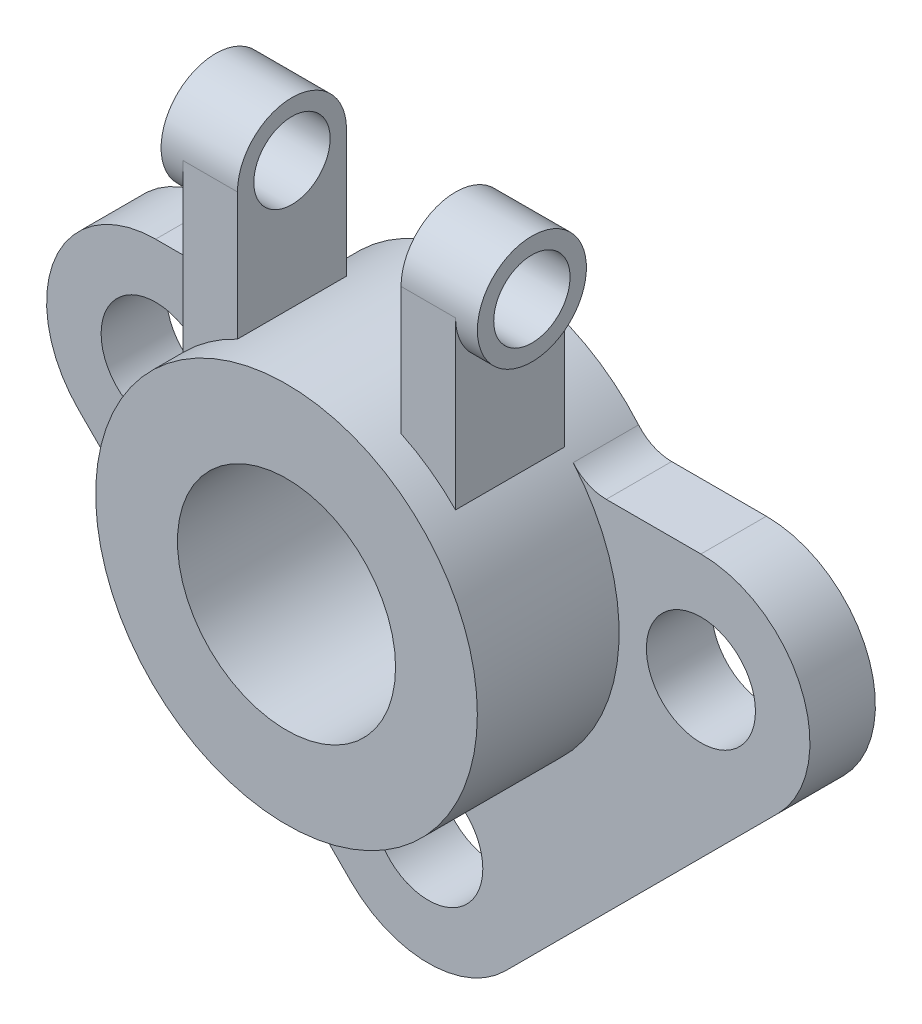
ISO-10303-21;
HEADER;
FILE_DESCRIPTION(('STEP AP214'),'2;1');
FILE_NAME('part.step','',(''),(''),'','','');
FILE_SCHEMA(('AUTOMOTIVE_DESIGN { 1 0 10303 214 1 1 1 1 }'));
ENDSEC;
DATA;
#1=APPLICATION_CONTEXT('core data for automotive mechanical design processes');
#2=APPLICATION_PROTOCOL_DEFINITION('international standard','automotive_design',2000,#1);
#3=PRODUCT_CONTEXT('',#1,'mechanical');
#4=PRODUCT('Part','Part','',(#3));
#5=PRODUCT_RELATED_PRODUCT_CATEGORY('part','',(#4));
#6=PRODUCT_DEFINITION_FORMATION('','',#4);
#7=PRODUCT_DEFINITION_CONTEXT('part definition',#1,'design');
#8=PRODUCT_DEFINITION('design','',#6,#7);
#9=PRODUCT_DEFINITION_SHAPE('','',#8);
#10=(LENGTH_UNIT() NAMED_UNIT(*) SI_UNIT(.MILLI.,.METRE.));
#11=(NAMED_UNIT(*) PLANE_ANGLE_UNIT() SI_UNIT($,.RADIAN.));
#12=(NAMED_UNIT(*) SI_UNIT($,.STERADIAN.) SOLID_ANGLE_UNIT());
#13=UNCERTAINTY_MEASURE_WITH_UNIT(LENGTH_MEASURE(1.E-05),#10,'distance_accuracy_value','');
#14=(GEOMETRIC_REPRESENTATION_CONTEXT(3) GLOBAL_UNCERTAINTY_ASSIGNED_CONTEXT((#13)) GLOBAL_UNIT_ASSIGNED_CONTEXT((#10,
#11,#12)) REPRESENTATION_CONTEXT('',''));
#15=CARTESIAN_POINT('',(0.,0.,0.));
#16=DIRECTION('',(0.,0.,1.));
#17=DIRECTION('',(1.,0.,0.));
#18=AXIS2_PLACEMENT_3D('',#15,#16,#17);
#19=CARTESIAN_POINT('',(0.,0.,38.));
#20=DIRECTION('',(0.,0.,-1.));
#21=DIRECTION('',(-1.,0.,0.));
#22=AXIS2_PLACEMENT_3D('',#19,#20,#21);
#23=CYLINDRICAL_SURFACE('',#22,35.);
#24=CARTESIAN_POINT('',(0.,0.,32.));
#25=DIRECTION('',(0.,0.,1.));
#26=DIRECTION('',(1.,0.,0.));
#27=AXIS2_PLACEMENT_3D('',#24,#25,#26);
#28=CIRCLE('',#27,35.);
#29=CARTESIAN_POINT('',(25.,24.4948974278318,32.));
#30=VERTEX_POINT('',#29);
#31=CARTESIAN_POINT('',(15.,31.6227766016838,32.));
#32=VERTEX_POINT('',#31);
#33=EDGE_CURVE('E309',#30,#32,#28,.T.);
#34=ORIENTED_EDGE('',*,*,#33,.T.);
#35=DIRECTION('',(0.,0.,-1.));
#36=VECTOR('',#35,1.);
#37=CARTESIAN_POINT('',(15.,31.6227766016838,38.));
#38=LINE('',#37,#36);
#39=CARTESIAN_POINT('',(15.,31.6227766016838,12.));
#40=VERTEX_POINT('',#39);
#41=EDGE_CURVE('E11',#32,#40,#38,.T.);
#42=ORIENTED_EDGE('',*,*,#41,.T.);
#43=CARTESIAN_POINT('',(0.,0.,12.));
#44=DIRECTION('',(0.,0.,-1.));
#45=DIRECTION('',(-1.,0.,0.));
#46=AXIS2_PLACEMENT_3D('',#43,#44,#45);
#47=CIRCLE('',#46,35.);
#48=CARTESIAN_POINT('',(25.,24.4948974278318,12.));
#49=VERTEX_POINT('',#48);
#50=EDGE_CURVE('E50',#40,#49,#47,.T.);
#51=ORIENTED_EDGE('',*,*,#50,.T.);
#52=DIRECTION('',(0.,0.,-1.));
#53=VECTOR('',#52,1.);
#54=CARTESIAN_POINT('',(25.,24.4948974278318,38.));
#55=LINE('',#54,#53);
#56=EDGE_CURVE('E311',#49,#30,#55,.F.);
#57=ORIENTED_EDGE('',*,*,#56,.T.);
#58=EDGE_LOOP('',(#34,#42,#51,#57));
#59=FACE_BOUND('',#58,.T.);
#60=CARTESIAN_POINT('',(0.,0.,12.));
#61=DIRECTION('',(0.,0.,-1.));
#62=DIRECTION('',(-1.,0.,0.));
#63=AXIS2_PLACEMENT_3D('',#60,#61,#62);
#64=CIRCLE('',#63,35.);
#65=CARTESIAN_POINT('',(-25.,24.4948974278318,12.));
#66=VERTEX_POINT('',#65);
#67=CARTESIAN_POINT('',(-15.,31.6227766016838,12.));
#68=VERTEX_POINT('',#67);
#69=EDGE_CURVE('E301',#66,#68,#64,.T.);
#70=ORIENTED_EDGE('',*,*,#69,.T.);
#71=DIRECTION('',(0.,0.,-1.));
#72=VECTOR('',#71,1.);
#73=CARTESIAN_POINT('',(-15.,31.6227766016838,38.));
#74=LINE('',#73,#72);
#75=CARTESIAN_POINT('',(-15.,31.6227766016838,32.));
#76=VERTEX_POINT('',#75);
#77=EDGE_CURVE('E177',#68,#76,#74,.F.);
#78=ORIENTED_EDGE('',*,*,#77,.T.);
#79=CARTESIAN_POINT('',(0.,0.,32.));
#80=DIRECTION('',(0.,0.,1.));
#81=DIRECTION('',(1.,0.,0.));
#82=AXIS2_PLACEMENT_3D('',#79,#80,#81);
#83=CIRCLE('',#82,35.);
#84=CARTESIAN_POINT('',(-25.,24.4948974278318,32.));
#85=VERTEX_POINT('',#84);
#86=EDGE_CURVE('E308',#76,#85,#83,.T.);
#87=ORIENTED_EDGE('',*,*,#86,.T.);
#88=DIRECTION('',(0.,0.,-1.));
#89=VECTOR('',#88,1.);
#90=CARTESIAN_POINT('',(-25.,24.4948974278318,38.));
#91=LINE('',#90,#89);
#92=EDGE_CURVE('E302',#85,#66,#91,.T.);
#93=ORIENTED_EDGE('',*,*,#92,.T.);
#94=EDGE_LOOP('',(#70,#78,#87,#93));
#95=FACE_BOUND('',#94,.T.);
#96=CARTESIAN_POINT('',(0.,0.,38.));
#97=DIRECTION('',(0.,0.,1.));
#98=DIRECTION('',(1.,0.,0.));
#99=AXIS2_PLACEMENT_3D('',#96,#97,#98);
#100=CIRCLE('',#99,35.);
#101=CARTESIAN_POINT('',(35.,0.,38.));
#102=VERTEX_POINT('',#101);
#103=EDGE_CURVE('E277',#102,#102,#100,.T.);
#104=ORIENTED_EDGE('',*,*,#103,.F.);
#105=EDGE_LOOP('',(#104));
#106=FACE_BOUND('',#105,.T.);
#107=CARTESIAN_POINT('',(0.,0.,0.));
#108=DIRECTION('',(0.,0.,1.));
#109=DIRECTION('',(1.,0.,0.));
#110=AXIS2_PLACEMENT_3D('',#107,#108,#109);
#111=CIRCLE('',#110,35.);
#112=CARTESIAN_POINT('',(26.5628330475733,22.7906976744186,0.));
#113=VERTEX_POINT('',#112);
#114=CARTESIAN_POINT('',(-26.5628330475733,22.7906976744186,0.));
#115=VERTEX_POINT('',#114);
#116=EDGE_CURVE('E272',#113,#115,#111,.T.);
#117=ORIENTED_EDGE('',*,*,#116,.T.);
#118=DIRECTION('',(0.,0.,-1.));
#119=VECTOR('',#118,1.);
#120=CARTESIAN_POINT('',(-26.5628330475733,22.7906976744186,38.));
#121=LINE('',#120,#119);
#122=CARTESIAN_POINT('',(-26.5628330475733,22.7906976744186,12.));
#123=VERTEX_POINT('',#122);
#124=EDGE_CURVE('E290',#115,#123,#121,.F.);
#125=ORIENTED_EDGE('',*,*,#124,.T.);
#126=CARTESIAN_POINT('',(0.,0.,12.));
#127=DIRECTION('',(0.,0.,-1.));
#128=DIRECTION('',(1.,0.,0.));
#129=AXIS2_PLACEMENT_3D('',#126,#127,#128);
#130=CIRCLE('',#129,35.);
#131=CARTESIAN_POINT('',(26.5628330475733,22.7906976744186,12.));
#132=VERTEX_POINT('',#131);
#133=EDGE_CURVE('E223',#132,#123,#130,.T.);
#134=ORIENTED_EDGE('',*,*,#133,.F.);
#135=DIRECTION('',(0.,0.,-1.));
#136=VECTOR('',#135,1.);
#137=CARTESIAN_POINT('',(26.5628330475733,22.7906976744186,38.));
#138=LINE('',#137,#136);
#139=EDGE_CURVE('E284',#132,#113,#138,.T.);
#140=ORIENTED_EDGE('',*,*,#139,.T.);
#141=EDGE_LOOP('',(#117,#125,#134,#140));
#142=FACE_BOUND('',#141,.T.);
#143=ADVANCED_FACE('F39',(#59,#95,#106,#142),#23,.T.);
#144=CARTESIAN_POINT('',(0.,0.,38.));
#145=DIRECTION('',(0.,0.,1.));
#146=DIRECTION('',(1.,0.,0.));
#147=AXIS2_PLACEMENT_3D('',#144,#145,#146);
#148=PLANE('',#147);
#149=ORIENTED_EDGE('',*,*,#103,.T.);
#150=EDGE_LOOP('',(#149));
#151=FACE_BOUND('',#150,.T.);
#152=CARTESIAN_POINT('',(0.,0.,38.));
#153=DIRECTION('',(0.,0.,1.));
#154=DIRECTION('',(1.,0.,0.));
#155=AXIS2_PLACEMENT_3D('',#152,#153,#154);
#156=CIRCLE('',#155,20.);
#157=CARTESIAN_POINT('',(20.,0.,38.));
#158=VERTEX_POINT('',#157);
#159=EDGE_CURVE('E269',#158,#158,#156,.T.);
#160=ORIENTED_EDGE('',*,*,#159,.F.);
#161=EDGE_LOOP('',(#160));
#162=FACE_BOUND('',#161,.T.);
#163=ADVANCED_FACE('F368',(#151,#162),#148,.T.);
#164=CARTESIAN_POINT('',(0.,0.,0.));
#165=DIRECTION('',(0.,0.,1.));
#166=DIRECTION('',(1.,0.,0.));
#167=AXIS2_PLACEMENT_3D('',#164,#165,#166);
#168=PLANE('',#167);
#169=ORIENTED_EDGE('',*,*,#116,.F.);
#170=CARTESIAN_POINT('',(32.6343377441615,28.,0.));
#171=DIRECTION('',(0.,0.,1.));
#172=DIRECTION('',(1.,0.,0.));
#173=AXIS2_PLACEMENT_3D('',#170,#171,#172);
#174=CIRCLE('',#173,8.);
#175=CARTESIAN_POINT('',(32.6343377441615,20.,0.));
#176=VERTEX_POINT('',#175);
#177=EDGE_CURVE('E297',#113,#176,#174,.T.);
#178=ORIENTED_EDGE('',*,*,#177,.T.);
#179=DIRECTION('',(-1.,0.,0.));
#180=VECTOR('',#179,1.);
#181=CARTESIAN_POINT('',(50.,20.,0.));
#182=LINE('',#181,#180);
#183=CARTESIAN_POINT('',(50.,20.,0.));
#184=VERTEX_POINT('',#183);
#185=EDGE_CURVE('E238',#184,#176,#182,.T.);
#186=ORIENTED_EDGE('',*,*,#185,.F.);
#187=CARTESIAN_POINT('',(50.,0.,0.));
#188=DIRECTION('',(0.,0.,1.));
#189=DIRECTION('',(1.,0.,0.));
#190=AXIS2_PLACEMENT_3D('',#187,#188,#189);
#191=CIRCLE('',#190,20.);
#192=CARTESIAN_POINT('',(64.142135623731,-14.1421356237309,0.));
#193=VERTEX_POINT('',#192);
#194=EDGE_CURVE('E214',#193,#184,#191,.T.);
#195=ORIENTED_EDGE('',*,*,#194,.F.);
#196=DIRECTION('',(0.707106781186547,0.707106781186548,0.));
#197=VECTOR('',#196,1.);
#198=CARTESIAN_POINT('',(14.142135623731,-64.142135623731,0.));
#199=LINE('',#198,#197);
#200=CARTESIAN_POINT('',(14.1421356237309,-64.142135623731,0.));
#201=VERTEX_POINT('',#200);
#202=EDGE_CURVE('E225',#201,#193,#199,.T.);
#203=ORIENTED_EDGE('',*,*,#202,.F.);
#204=CARTESIAN_POINT('',(0.,-50.,0.));
#205=DIRECTION('',(0.,0.,1.));
#206=DIRECTION('',(1.,0.,0.));
#207=AXIS2_PLACEMENT_3D('',#204,#205,#206);
#208=CIRCLE('',#207,20.);
#209=CARTESIAN_POINT('',(-14.142135623731,-64.142135623731,0.));
#210=VERTEX_POINT('',#209);
#211=EDGE_CURVE('E248',#210,#201,#208,.T.);
#212=ORIENTED_EDGE('',*,*,#211,.F.);
#213=DIRECTION('',(0.707106781186547,-0.707106781186547,0.));
#214=VECTOR('',#213,1.);
#215=CARTESIAN_POINT('',(-64.142135623731,-14.142135623731,0.));
#216=LINE('',#215,#214);
#217=CARTESIAN_POINT('',(-64.142135623731,-14.142135623731,0.));
#218=VERTEX_POINT('',#217);
#219=EDGE_CURVE('E250',#218,#210,#216,.T.);
#220=ORIENTED_EDGE('',*,*,#219,.F.);
#221=CARTESIAN_POINT('',(-50.,0.,0.));
#222=DIRECTION('',(0.,0.,1.));
#223=DIRECTION('',(-1.,0.,0.));
#224=AXIS2_PLACEMENT_3D('',#221,#222,#223);
#225=CIRCLE('',#224,20.);
#226=CARTESIAN_POINT('',(-50.,20.,0.));
#227=VERTEX_POINT('',#226);
#228=EDGE_CURVE('E241',#227,#218,#225,.T.);
#229=ORIENTED_EDGE('',*,*,#228,.F.);
#230=DIRECTION('',(-1.,0.,0.));
#231=VECTOR('',#230,1.);
#232=CARTESIAN_POINT('',(-50.,20.,0.));
#233=LINE('',#232,#231);
#234=CARTESIAN_POINT('',(-32.6343377441615,20.,0.));
#235=VERTEX_POINT('',#234);
#236=EDGE_CURVE('E243',#235,#227,#233,.T.);
#237=ORIENTED_EDGE('',*,*,#236,.F.);
#238=CARTESIAN_POINT('',(-32.6343377441615,28.,0.));
#239=DIRECTION('',(0.,0.,1.));
#240=DIRECTION('',(1.,0.,0.));
#241=AXIS2_PLACEMENT_3D('',#238,#239,#240);
#242=CIRCLE('',#241,8.);
#243=EDGE_CURVE('E295',#235,#115,#242,.T.);
#244=ORIENTED_EDGE('',*,*,#243,.T.);
#245=EDGE_LOOP('',(#169,#178,#186,#195,#203,#212,#220,#229,#237,#244));
#246=FACE_BOUND('',#245,.T.);
#247=CARTESIAN_POINT('',(0.,0.,0.));
#248=DIRECTION('',(0.,0.,1.));
#249=DIRECTION('',(1.,0.,0.));
#250=AXIS2_PLACEMENT_3D('',#247,#248,#249);
#251=CIRCLE('',#250,20.);
#252=CARTESIAN_POINT('',(20.,0.,0.));
#253=VERTEX_POINT('',#252);
#254=EDGE_CURVE('E267',#253,#253,#251,.T.);
#255=ORIENTED_EDGE('',*,*,#254,.T.);
#256=EDGE_LOOP('',(#255));
#257=FACE_BOUND('',#256,.T.);
#258=CARTESIAN_POINT('',(50.,0.,0.));
#259=DIRECTION('',(0.,0.,1.));
#260=DIRECTION('',(1.,0.,0.));
#261=AXIS2_PLACEMENT_3D('',#258,#259,#260);
#262=CIRCLE('',#261,10.);
#263=CARTESIAN_POINT('',(60.,0.,0.));
#264=VERTEX_POINT('',#263);
#265=EDGE_CURVE('E207',#264,#264,#262,.T.);
#266=ORIENTED_EDGE('',*,*,#265,.T.);
#267=EDGE_LOOP('',(#266));
#268=FACE_BOUND('',#267,.T.);
#269=CARTESIAN_POINT('',(0.,-50.,0.));
#270=DIRECTION('',(0.,0.,1.));
#271=DIRECTION('',(1.,0.,0.));
#272=AXIS2_PLACEMENT_3D('',#269,#270,#271);
#273=CIRCLE('',#272,10.);
#274=CARTESIAN_POINT('',(10.,-50.,0.));
#275=VERTEX_POINT('',#274);
#276=EDGE_CURVE('E201',#275,#275,#273,.T.);
#277=ORIENTED_EDGE('',*,*,#276,.T.);
#278=EDGE_LOOP('',(#277));
#279=FACE_BOUND('',#278,.T.);
#280=CARTESIAN_POINT('',(-50.,0.,0.));
#281=DIRECTION('',(0.,0.,1.));
#282=DIRECTION('',(-1.,0.,0.));
#283=AXIS2_PLACEMENT_3D('',#280,#281,#282);
#284=CIRCLE('',#283,10.);
#285=CARTESIAN_POINT('',(-60.,0.,0.));
#286=VERTEX_POINT('',#285);
#287=EDGE_CURVE('E194',#286,#286,#284,.T.);
#288=ORIENTED_EDGE('',*,*,#287,.T.);
#289=EDGE_LOOP('',(#288));
#290=FACE_BOUND('',#289,.T.);
#291=ADVANCED_FACE('F375',(#246,#257,#268,#279,#290),#168,.F.);
#292=CARTESIAN_POINT('',(0.,0.,38.));
#293=DIRECTION('',(0.,0.,-1.));
#294=DIRECTION('',(-1.,0.,0.));
#295=AXIS2_PLACEMENT_3D('',#292,#293,#294);
#296=CYLINDRICAL_SURFACE('',#295,20.);
#297=ORIENTED_EDGE('',*,*,#159,.T.);
#298=EDGE_LOOP('',(#297));
#299=FACE_BOUND('',#298,.T.);
#300=ORIENTED_EDGE('',*,*,#254,.F.);
#301=EDGE_LOOP('',(#300));
#302=FACE_BOUND('',#301,.T.);
#303=ADVANCED_FACE('F432',(#299,#302),#296,.F.);
#304=CARTESIAN_POINT('',(50.,0.,12.));
#305=DIRECTION('',(0.,0.,1.));
#306=DIRECTION('',(1.,0.,0.));
#307=AXIS2_PLACEMENT_3D('',#304,#305,#306);
#308=PLANE('',#307);
#309=CARTESIAN_POINT('',(0.,-50.,12.));
#310=DIRECTION('',(0.,0.,1.));
#311=DIRECTION('',(1.,0.,0.));
#312=AXIS2_PLACEMENT_3D('',#309,#310,#311);
#313=CIRCLE('',#312,10.);
#314=CARTESIAN_POINT('',(10.,-50.,12.));
#315=VERTEX_POINT('',#314);
#316=EDGE_CURVE('E206',#315,#315,#313,.T.);
#317=ORIENTED_EDGE('',*,*,#316,.F.);
#318=EDGE_LOOP('',(#317));
#319=FACE_BOUND('',#318,.T.);
#320=CARTESIAN_POINT('',(50.,0.,12.));
#321=DIRECTION('',(0.,0.,1.));
#322=DIRECTION('',(1.,0.,0.));
#323=AXIS2_PLACEMENT_3D('',#320,#321,#322);
#324=CIRCLE('',#323,20.);
#325=CARTESIAN_POINT('',(64.142135623731,-14.1421356237309,12.));
#326=VERTEX_POINT('',#325);
#327=CARTESIAN_POINT('',(50.,20.,12.));
#328=VERTEX_POINT('',#327);
#329=EDGE_CURVE('E217',#326,#328,#324,.T.);
#330=ORIENTED_EDGE('',*,*,#329,.T.);
#331=DIRECTION('',(-1.,0.,0.));
#332=VECTOR('',#331,1.);
#333=CARTESIAN_POINT('',(50.,20.,12.));
#334=LINE('',#333,#332);
#335=CARTESIAN_POINT('',(32.6343377441615,20.,12.));
#336=VERTEX_POINT('',#335);
#337=EDGE_CURVE('E222',#328,#336,#334,.T.);
#338=ORIENTED_EDGE('',*,*,#337,.T.);
#339=CARTESIAN_POINT('',(32.6343377441615,28.,12.));
#340=DIRECTION('',(0.,0.,1.));
#341=DIRECTION('',(1.,0.,0.));
#342=AXIS2_PLACEMENT_3D('',#339,#340,#341);
#343=CIRCLE('',#342,8.);
#344=EDGE_CURVE('E298',#336,#132,#343,.F.);
#345=ORIENTED_EDGE('',*,*,#344,.T.);
#346=ORIENTED_EDGE('',*,*,#133,.T.);
#347=CARTESIAN_POINT('',(-32.6343377441615,28.,12.));
#348=DIRECTION('',(0.,0.,1.));
#349=DIRECTION('',(1.,0.,0.));
#350=AXIS2_PLACEMENT_3D('',#347,#348,#349);
#351=CIRCLE('',#350,8.);
#352=CARTESIAN_POINT('',(-32.6343377441615,20.,12.));
#353=VERTEX_POINT('',#352);
#354=EDGE_CURVE('E294',#123,#353,#351,.F.);
#355=ORIENTED_EDGE('',*,*,#354,.T.);
#356=DIRECTION('',(-1.,0.,0.));
#357=VECTOR('',#356,1.);
#358=CARTESIAN_POINT('',(-50.,20.,12.));
#359=LINE('',#358,#357);
#360=CARTESIAN_POINT('',(-50.,20.,12.));
#361=VERTEX_POINT('',#360);
#362=EDGE_CURVE('E230',#353,#361,#359,.T.);
#363=ORIENTED_EDGE('',*,*,#362,.T.);
#364=CARTESIAN_POINT('',(-50.,0.,12.));
#365=DIRECTION('',(0.,0.,1.));
#366=DIRECTION('',(-1.,0.,0.));
#367=AXIS2_PLACEMENT_3D('',#364,#365,#366);
#368=CIRCLE('',#367,20.);
#369=CARTESIAN_POINT('',(-64.142135623731,-14.142135623731,12.));
#370=VERTEX_POINT('',#369);
#371=EDGE_CURVE('E229',#361,#370,#368,.T.);
#372=ORIENTED_EDGE('',*,*,#371,.T.);
#373=DIRECTION('',(0.707106781186547,-0.707106781186547,0.));
#374=VECTOR('',#373,1.);
#375=CARTESIAN_POINT('',(-64.142135623731,-14.142135623731,12.));
#376=LINE('',#375,#374);
#377=CARTESIAN_POINT('',(-14.142135623731,-64.142135623731,12.));
#378=VERTEX_POINT('',#377);
#379=EDGE_CURVE('E231',#370,#378,#376,.T.);
#380=ORIENTED_EDGE('',*,*,#379,.T.);
#381=CARTESIAN_POINT('',(0.,-50.,12.));
#382=DIRECTION('',(0.,0.,1.));
#383=DIRECTION('',(1.,0.,0.));
#384=AXIS2_PLACEMENT_3D('',#381,#382,#383);
#385=CIRCLE('',#384,20.);
#386=CARTESIAN_POINT('',(14.1421356237309,-64.142135623731,12.));
#387=VERTEX_POINT('',#386);
#388=EDGE_CURVE('E232',#378,#387,#385,.T.);
#389=ORIENTED_EDGE('',*,*,#388,.T.);
#390=DIRECTION('',(0.707106781186547,0.707106781186548,0.));
#391=VECTOR('',#390,1.);
#392=CARTESIAN_POINT('',(14.142135623731,-64.142135623731,12.));
#393=LINE('',#392,#391);
#394=EDGE_CURVE('E234',#387,#326,#393,.T.);
#395=ORIENTED_EDGE('',*,*,#394,.T.);
#396=EDGE_LOOP('',(#330,#338,#345,#346,#355,#363,#372,#380,#389,#395));
#397=FACE_BOUND('',#396,.T.);
#398=CARTESIAN_POINT('',(50.,0.,12.));
#399=DIRECTION('',(0.,0.,1.));
#400=DIRECTION('',(1.,0.,0.));
#401=AXIS2_PLACEMENT_3D('',#398,#399,#400);
#402=CIRCLE('',#401,10.);
#403=CARTESIAN_POINT('',(60.,0.,12.));
#404=VERTEX_POINT('',#403);
#405=EDGE_CURVE('E215',#404,#404,#402,.T.);
#406=ORIENTED_EDGE('',*,*,#405,.F.);
#407=EDGE_LOOP('',(#406));
#408=FACE_BOUND('',#407,.T.);
#409=CARTESIAN_POINT('',(-50.,0.,12.));
#410=DIRECTION('',(0.,0.,1.));
#411=DIRECTION('',(-1.,0.,0.));
#412=AXIS2_PLACEMENT_3D('',#409,#410,#411);
#413=CIRCLE('',#412,10.);
#414=CARTESIAN_POINT('',(-60.,0.,12.));
#415=VERTEX_POINT('',#414);
#416=EDGE_CURVE('E199',#415,#415,#413,.T.);
#417=ORIENTED_EDGE('',*,*,#416,.F.);
#418=EDGE_LOOP('',(#417));
#419=FACE_BOUND('',#418,.T.);
#420=ADVANCED_FACE('F393',(#319,#397,#408,#419),#308,.T.);
#421=CARTESIAN_POINT('',(50.,0.,12.));
#422=DIRECTION('',(0.,0.,-1.));
#423=DIRECTION('',(-1.,0.,0.));
#424=AXIS2_PLACEMENT_3D('',#421,#422,#423);
#425=CYLINDRICAL_SURFACE('',#424,20.);
#426=ORIENTED_EDGE('',*,*,#194,.T.);
#427=DIRECTION('',(0.,0.,-1.));
#428=VECTOR('',#427,1.);
#429=CARTESIAN_POINT('',(50.,20.,12.));
#430=LINE('',#429,#428);
#431=EDGE_CURVE('E266',#328,#184,#430,.T.);
#432=ORIENTED_EDGE('',*,*,#431,.F.);
#433=ORIENTED_EDGE('',*,*,#329,.F.);
#434=DIRECTION('',(0.,0.,-1.));
#435=VECTOR('',#434,1.);
#436=CARTESIAN_POINT('',(64.142135623731,-14.1421356237309,12.));
#437=LINE('',#436,#435);
#438=EDGE_CURVE('E240',#326,#193,#437,.T.);
#439=ORIENTED_EDGE('',*,*,#438,.T.);
#440=EDGE_LOOP('',(#426,#432,#433,#439));
#441=FACE_BOUND('',#440,.T.);
#442=ADVANCED_FACE('F421',(#441),#425,.T.);
#443=CARTESIAN_POINT('',(50.,20.,12.));
#444=DIRECTION('',(0.,-1.,0.));
#445=DIRECTION('',(0.,0.,-1.));
#446=AXIS2_PLACEMENT_3D('',#443,#444,#445);
#447=PLANE('',#446);
#448=ORIENTED_EDGE('',*,*,#185,.T.);
#449=DIRECTION('',(0.,0.,1.));
#450=VECTOR('',#449,1.);
#451=CARTESIAN_POINT('',(32.6343377441615,20.,12.));
#452=LINE('',#451,#450);
#453=EDGE_CURVE('E289',#176,#336,#452,.T.);
#454=ORIENTED_EDGE('',*,*,#453,.T.);
#455=ORIENTED_EDGE('',*,*,#337,.F.);
#456=ORIENTED_EDGE('',*,*,#431,.T.);
#457=EDGE_LOOP('',(#448,#454,#455,#456));
#458=FACE_BOUND('',#457,.T.);
#459=ADVANCED_FACE('F426',(#458),#447,.F.);
#460=CARTESIAN_POINT('',(-50.,20.,12.));
#461=DIRECTION('',(0.,-1.,0.));
#462=DIRECTION('',(1.,0.,0.));
#463=AXIS2_PLACEMENT_3D('',#460,#461,#462);
#464=PLANE('',#463);
#465=ORIENTED_EDGE('',*,*,#362,.F.);
#466=DIRECTION('',(0.,0.,1.));
#467=VECTOR('',#466,1.);
#468=CARTESIAN_POINT('',(-32.6343377441615,20.,0.));
#469=LINE('',#468,#467);
#470=EDGE_CURVE('E276',#353,#235,#469,.F.);
#471=ORIENTED_EDGE('',*,*,#470,.T.);
#472=ORIENTED_EDGE('',*,*,#236,.T.);
#473=DIRECTION('',(0.,0.,-1.));
#474=VECTOR('',#473,1.);
#475=CARTESIAN_POINT('',(-50.,20.,12.));
#476=LINE('',#475,#474);
#477=EDGE_CURVE('E263',#361,#227,#476,.T.);
#478=ORIENTED_EDGE('',*,*,#477,.F.);
#479=EDGE_LOOP('',(#465,#471,#472,#478));
#480=FACE_BOUND('',#479,.T.);
#481=ADVANCED_FACE('F400',(#480),#464,.F.);
#482=CARTESIAN_POINT('',(-50.,0.,12.));
#483=DIRECTION('',(0.,0.,-1.));
#484=DIRECTION('',(-1.,0.,0.));
#485=AXIS2_PLACEMENT_3D('',#482,#483,#484);
#486=CYLINDRICAL_SURFACE('',#485,20.);
#487=ORIENTED_EDGE('',*,*,#228,.T.);
#488=DIRECTION('',(0.,0.,-1.));
#489=VECTOR('',#488,1.);
#490=CARTESIAN_POINT('',(-64.142135623731,-14.142135623731,12.));
#491=LINE('',#490,#489);
#492=EDGE_CURVE('E257',#370,#218,#491,.T.);
#493=ORIENTED_EDGE('',*,*,#492,.F.);
#494=ORIENTED_EDGE('',*,*,#371,.F.);
#495=ORIENTED_EDGE('',*,*,#477,.T.);
#496=EDGE_LOOP('',(#487,#493,#494,#495));
#497=FACE_BOUND('',#496,.T.);
#498=ADVANCED_FACE('F401',(#497),#486,.T.);
#499=CARTESIAN_POINT('',(-64.142135623731,-14.142135623731,12.));
#500=DIRECTION('',(0.707106781186548,0.707106781186548,0.));
#501=DIRECTION('',(-0.707106781186548,0.707106781186548,0.));
#502=AXIS2_PLACEMENT_3D('',#499,#500,#501);
#503=PLANE('',#502);
#504=ORIENTED_EDGE('',*,*,#219,.T.);
#505=DIRECTION('',(0.,0.,-1.));
#506=VECTOR('',#505,1.);
#507=CARTESIAN_POINT('',(-14.142135623731,-64.142135623731,12.));
#508=LINE('',#507,#506);
#509=EDGE_CURVE('E260',#378,#210,#508,.T.);
#510=ORIENTED_EDGE('',*,*,#509,.F.);
#511=ORIENTED_EDGE('',*,*,#379,.F.);
#512=ORIENTED_EDGE('',*,*,#492,.T.);
#513=EDGE_LOOP('',(#504,#510,#511,#512));
#514=FACE_BOUND('',#513,.T.);
#515=ADVANCED_FACE('F409',(#514),#503,.F.);
#516=CARTESIAN_POINT('',(0.,-50.,12.));
#517=DIRECTION('',(0.,0.,-1.));
#518=DIRECTION('',(-1.,0.,0.));
#519=AXIS2_PLACEMENT_3D('',#516,#517,#518);
#520=CYLINDRICAL_SURFACE('',#519,20.);
#521=ORIENTED_EDGE('',*,*,#211,.T.);
#522=DIRECTION('',(0.,0.,-1.));
#523=VECTOR('',#522,1.);
#524=CARTESIAN_POINT('',(14.1421356237309,-64.142135623731,12.));
#525=LINE('',#524,#523);
#526=EDGE_CURVE('E255',#387,#201,#525,.T.);
#527=ORIENTED_EDGE('',*,*,#526,.F.);
#528=ORIENTED_EDGE('',*,*,#388,.F.);
#529=ORIENTED_EDGE('',*,*,#509,.T.);
#530=EDGE_LOOP('',(#521,#527,#528,#529));
#531=FACE_BOUND('',#530,.T.);
#532=ADVANCED_FACE('F412',(#531),#520,.T.);
#533=CARTESIAN_POINT('',(14.142135623731,-64.142135623731,12.));
#534=DIRECTION('',(-0.707106781186548,0.707106781186547,0.));
#535=DIRECTION('',(-0.707106781186547,-0.707106781186548,0.));
#536=AXIS2_PLACEMENT_3D('',#533,#534,#535);
#537=PLANE('',#536);
#538=ORIENTED_EDGE('',*,*,#202,.T.);
#539=ORIENTED_EDGE('',*,*,#438,.F.);
#540=ORIENTED_EDGE('',*,*,#394,.F.);
#541=ORIENTED_EDGE('',*,*,#526,.T.);
#542=EDGE_LOOP('',(#538,#539,#540,#541));
#543=FACE_BOUND('',#542,.T.);
#544=ADVANCED_FACE('F416',(#543),#537,.F.);
#545=CARTESIAN_POINT('',(50.,0.,12.));
#546=DIRECTION('',(0.,0.,-1.));
#547=DIRECTION('',(-1.,0.,0.));
#548=AXIS2_PLACEMENT_3D('',#545,#546,#547);
#549=CYLINDRICAL_SURFACE('',#548,10.);
#550=ORIENTED_EDGE('',*,*,#405,.T.);
#551=EDGE_LOOP('',(#550));
#552=FACE_BOUND('',#551,.T.);
#553=ORIENTED_EDGE('',*,*,#265,.F.);
#554=EDGE_LOOP('',(#553));
#555=FACE_BOUND('',#554,.T.);
#556=ADVANCED_FACE('F443',(#552,#555),#549,.F.);
#557=CARTESIAN_POINT('',(0.,-50.,12.));
#558=DIRECTION('',(0.,0.,-1.));
#559=DIRECTION('',(-1.,0.,0.));
#560=AXIS2_PLACEMENT_3D('',#557,#558,#559);
#561=CYLINDRICAL_SURFACE('',#560,10.);
#562=ORIENTED_EDGE('',*,*,#316,.T.);
#563=EDGE_LOOP('',(#562));
#564=FACE_BOUND('',#563,.T.);
#565=ORIENTED_EDGE('',*,*,#276,.F.);
#566=EDGE_LOOP('',(#565));
#567=FACE_BOUND('',#566,.T.);
#568=ADVANCED_FACE('F384',(#564,#567),#561,.F.);
#569=CARTESIAN_POINT('',(-50.,0.,12.));
#570=DIRECTION('',(0.,0.,-1.));
#571=DIRECTION('',(-1.,0.,0.));
#572=AXIS2_PLACEMENT_3D('',#569,#570,#571);
#573=CYLINDRICAL_SURFACE('',#572,10.);
#574=ORIENTED_EDGE('',*,*,#416,.T.);
#575=EDGE_LOOP('',(#574));
#576=FACE_BOUND('',#575,.T.);
#577=ORIENTED_EDGE('',*,*,#287,.F.);
#578=EDGE_LOOP('',(#577));
#579=FACE_BOUND('',#578,.T.);
#580=ADVANCED_FACE('F378',(#576,#579),#573,.F.);
#581=CARTESIAN_POINT('',(-32.6343377441615,28.,38.));
#582=DIRECTION('',(0.,0.,-1.));
#583=DIRECTION('',(-1.,0.,0.));
#584=AXIS2_PLACEMENT_3D('',#581,#582,#583);
#585=CYLINDRICAL_SURFACE('',#584,8.);
#586=ORIENTED_EDGE('',*,*,#354,.F.);
#587=ORIENTED_EDGE('',*,*,#124,.F.);
#588=ORIENTED_EDGE('',*,*,#243,.F.);
#589=ORIENTED_EDGE('',*,*,#470,.F.);
#590=EDGE_LOOP('',(#586,#587,#588,#589));
#591=FACE_BOUND('',#590,.T.);
#592=ADVANCED_FACE('F376',(#591),#585,.F.);
#593=CARTESIAN_POINT('',(32.6343377441615,28.,38.));
#594=DIRECTION('',(0.,0.,-1.));
#595=DIRECTION('',(-1.,0.,0.));
#596=AXIS2_PLACEMENT_3D('',#593,#594,#595);
#597=CYLINDRICAL_SURFACE('',#596,8.);
#598=ORIENTED_EDGE('',*,*,#344,.F.);
#599=ORIENTED_EDGE('',*,*,#453,.F.);
#600=ORIENTED_EDGE('',*,*,#177,.F.);
#601=ORIENTED_EDGE('',*,*,#139,.F.);
#602=EDGE_LOOP('',(#598,#599,#600,#601));
#603=FACE_BOUND('',#602,.T.);
#604=ADVANCED_FACE('F41',(#603),#597,.F.);
#605=CARTESIAN_POINT('',(-15.,23.,32.));
#606=DIRECTION('',(1.,0.,0.));
#607=DIRECTION('',(0.,0.,-1.));
#608=AXIS2_PLACEMENT_3D('',#605,#606,#607);
#609=PLANE('',#608);
#610=CARTESIAN_POINT('',(-15.,55.,22.));
#611=DIRECTION('',(1.,0.,0.));
#612=DIRECTION('',(0.,0.,-1.));
#613=AXIS2_PLACEMENT_3D('',#610,#611,#612);
#614=CIRCLE('',#613,6.99999999999999);
#615=CARTESIAN_POINT('',(-15.,55.,15.));
#616=VERTEX_POINT('',#615);
#617=EDGE_CURVE('E675',#616,#616,#614,.T.);
#618=ORIENTED_EDGE('',*,*,#617,.F.);
#619=EDGE_LOOP('',(#618));
#620=FACE_BOUND('',#619,.T.);
#621=DIRECTION('',(0.,1.,0.));
#622=VECTOR('',#621,1.);
#623=CARTESIAN_POINT('',(-15.,23.,12.));
#624=LINE('',#623,#622);
#625=CARTESIAN_POINT('',(-15.,55.,12.));
#626=VERTEX_POINT('',#625);
#627=EDGE_CURVE('E65',#68,#626,#624,.T.);
#628=ORIENTED_EDGE('',*,*,#627,.T.);
#629=CARTESIAN_POINT('',(-15.,55.,22.));
#630=DIRECTION('',(1.,0.,0.));
#631=DIRECTION('',(0.,0.,-1.));
#632=AXIS2_PLACEMENT_3D('',#629,#630,#631);
#633=CIRCLE('',#632,10.);
#634=CARTESIAN_POINT('',(-15.,55.,32.));
#635=VERTEX_POINT('',#634);
#636=EDGE_CURVE('E163',#626,#635,#633,.T.);
#637=ORIENTED_EDGE('',*,*,#636,.T.);
#638=DIRECTION('',(0.,1.,0.));
#639=VECTOR('',#638,1.);
#640=CARTESIAN_POINT('',(-15.,23.,32.));
#641=LINE('',#640,#639);
#642=EDGE_CURVE('E192',#76,#635,#641,.T.);
#643=ORIENTED_EDGE('',*,*,#642,.F.);
#644=ORIENTED_EDGE('',*,*,#77,.F.);
#645=EDGE_LOOP('',(#628,#637,#643,#644));
#646=FACE_BOUND('',#645,.T.);
#647=ADVANCED_FACE('F176',(#620,#646),#609,.T.);
#648=CARTESIAN_POINT('',(-25.,23.,32.));
#649=DIRECTION('',(-1.,0.,0.));
#650=DIRECTION('',(0.,0.,1.));
#651=AXIS2_PLACEMENT_3D('',#648,#649,#650);
#652=PLANE('',#651);
#653=CARTESIAN_POINT('',(-25.,55.,22.));
#654=DIRECTION('',(-1.,0.,0.));
#655=DIRECTION('',(0.,0.,1.));
#656=AXIS2_PLACEMENT_3D('',#653,#654,#655);
#657=CIRCLE('',#656,10.);
#658=CARTESIAN_POINT('',(-25.,55.,12.));
#659=VERTEX_POINT('',#658);
#660=CARTESIAN_POINT('',(-25.,55.,32.));
#661=VERTEX_POINT('',#660);
#662=EDGE_CURVE('E666',#659,#661,#657,.T.);
#663=ORIENTED_EDGE('',*,*,#662,.F.);
#664=DIRECTION('',(0.,1.,0.));
#665=VECTOR('',#664,1.);
#666=CARTESIAN_POINT('',(-25.,23.,12.));
#667=LINE('',#666,#665);
#668=EDGE_CURVE('E179',#66,#659,#667,.T.);
#669=ORIENTED_EDGE('',*,*,#668,.F.);
#670=ORIENTED_EDGE('',*,*,#92,.F.);
#671=DIRECTION('',(0.,1.,0.));
#672=VECTOR('',#671,1.);
#673=CARTESIAN_POINT('',(-25.,23.,32.));
#674=LINE('',#673,#672);
#675=EDGE_CURVE('E198',#85,#661,#674,.T.);
#676=ORIENTED_EDGE('',*,*,#675,.T.);
#677=EDGE_LOOP('',(#663,#669,#670,#676));
#678=FACE_BOUND('',#677,.T.);
#679=ADVANCED_FACE('F546',(#678),#652,.T.);
#680=CARTESIAN_POINT('',(-15.,23.,32.));
#681=DIRECTION('',(0.,0.,1.));
#682=DIRECTION('',(1.,0.,0.));
#683=AXIS2_PLACEMENT_3D('',#680,#681,#682);
#684=PLANE('',#683);
#685=ORIENTED_EDGE('',*,*,#86,.F.);
#686=ORIENTED_EDGE('',*,*,#642,.T.);
#687=DIRECTION('',(1.,0.,0.));
#688=VECTOR('',#687,1.);
#689=CARTESIAN_POINT('',(-15.,55.,32.));
#690=LINE('',#689,#688);
#691=EDGE_CURVE('E166',#661,#635,#690,.T.);
#692=ORIENTED_EDGE('',*,*,#691,.F.);
#693=ORIENTED_EDGE('',*,*,#675,.F.);
#694=EDGE_LOOP('',(#685,#686,#692,#693));
#695=FACE_BOUND('',#694,.T.);
#696=ADVANCED_FACE('F558',(#695),#684,.T.);
#697=CARTESIAN_POINT('',(-15.,23.,12.));
#698=DIRECTION('',(0.,0.,-1.));
#699=DIRECTION('',(-1.,0.,0.));
#700=AXIS2_PLACEMENT_3D('',#697,#698,#699);
#701=PLANE('',#700);
#702=ORIENTED_EDGE('',*,*,#69,.F.);
#703=ORIENTED_EDGE('',*,*,#668,.T.);
#704=DIRECTION('',(-1.,0.,0.));
#705=VECTOR('',#704,1.);
#706=CARTESIAN_POINT('',(-15.,55.,12.));
#707=LINE('',#706,#705);
#708=EDGE_CURVE('E167',#626,#659,#707,.T.);
#709=ORIENTED_EDGE('',*,*,#708,.F.);
#710=ORIENTED_EDGE('',*,*,#627,.F.);
#711=EDGE_LOOP('',(#702,#703,#709,#710));
#712=FACE_BOUND('',#711,.T.);
#713=ADVANCED_FACE('F181',(#712),#701,.T.);
#714=CARTESIAN_POINT('',(15.,23.,32.));
#715=DIRECTION('',(-1.,0.,0.));
#716=DIRECTION('',(0.,0.,1.));
#717=AXIS2_PLACEMENT_3D('',#714,#715,#716);
#718=PLANE('',#717);
#719=CARTESIAN_POINT('',(15.,55.,22.));
#720=DIRECTION('',(-1.,0.,0.));
#721=DIRECTION('',(0.,0.,1.));
#722=AXIS2_PLACEMENT_3D('',#719,#720,#721);
#723=CIRCLE('',#722,7.);
#724=CARTESIAN_POINT('',(15.,55.,29.));
#725=VERTEX_POINT('',#724);
#726=EDGE_CURVE('E338',#725,#725,#723,.T.);
#727=ORIENTED_EDGE('',*,*,#726,.F.);
#728=EDGE_LOOP('',(#727));
#729=FACE_BOUND('',#728,.T.);
#730=DIRECTION('',(0.,1.,0.));
#731=VECTOR('',#730,1.);
#732=CARTESIAN_POINT('',(15.,23.,32.));
#733=LINE('',#732,#731);
#734=CARTESIAN_POINT('',(15.,55.,32.));
#735=VERTEX_POINT('',#734);
#736=EDGE_CURVE('E53',#32,#735,#733,.T.);
#737=ORIENTED_EDGE('',*,*,#736,.T.);
#738=CARTESIAN_POINT('',(15.,55.,22.));
#739=DIRECTION('',(-1.,0.,0.));
#740=DIRECTION('',(0.,0.,1.));
#741=AXIS2_PLACEMENT_3D('',#738,#739,#740);
#742=CIRCLE('',#741,9.99999999999999);
#743=CARTESIAN_POINT('',(15.,55.,12.));
#744=VERTEX_POINT('',#743);
#745=EDGE_CURVE('E327',#735,#744,#742,.T.);
#746=ORIENTED_EDGE('',*,*,#745,.T.);
#747=DIRECTION('',(0.,1.,0.));
#748=VECTOR('',#747,1.);
#749=CARTESIAN_POINT('',(15.,23.,12.));
#750=LINE('',#749,#748);
#751=EDGE_CURVE('E183',#40,#744,#750,.T.);
#752=ORIENTED_EDGE('',*,*,#751,.F.);
#753=ORIENTED_EDGE('',*,*,#41,.F.);
#754=EDGE_LOOP('',(#737,#746,#752,#753));
#755=FACE_BOUND('',#754,.T.);
#756=ADVANCED_FACE('F326',(#729,#755),#718,.T.);
#757=CARTESIAN_POINT('',(25.,23.,32.));
#758=DIRECTION('',(1.,0.,0.));
#759=DIRECTION('',(0.,0.,-1.));
#760=AXIS2_PLACEMENT_3D('',#757,#758,#759);
#761=PLANE('',#760);
#762=CARTESIAN_POINT('',(25.,55.,22.));
#763=DIRECTION('',(1.,0.,0.));
#764=DIRECTION('',(0.,0.,-1.));
#765=AXIS2_PLACEMENT_3D('',#762,#763,#764);
#766=CIRCLE('',#765,9.99999999999999);
#767=CARTESIAN_POINT('',(25.,55.,32.));
#768=VERTEX_POINT('',#767);
#769=CARTESIAN_POINT('',(25.,55.,12.));
#770=VERTEX_POINT('',#769);
#771=EDGE_CURVE('E333',#768,#770,#766,.T.);
#772=ORIENTED_EDGE('',*,*,#771,.F.);
#773=DIRECTION('',(0.,1.,0.));
#774=VECTOR('',#773,1.);
#775=CARTESIAN_POINT('',(25.,23.,32.));
#776=LINE('',#775,#774);
#777=EDGE_CURVE('E346',#30,#768,#776,.T.);
#778=ORIENTED_EDGE('',*,*,#777,.F.);
#779=ORIENTED_EDGE('',*,*,#56,.F.);
#780=DIRECTION('',(0.,1.,0.));
#781=VECTOR('',#780,1.);
#782=CARTESIAN_POINT('',(25.,23.,12.));
#783=LINE('',#782,#781);
#784=EDGE_CURVE('E188',#49,#770,#783,.T.);
#785=ORIENTED_EDGE('',*,*,#784,.T.);
#786=EDGE_LOOP('',(#772,#778,#779,#785));
#787=FACE_BOUND('',#786,.T.);
#788=ADVANCED_FACE('F354',(#787),#761,.T.);
#789=CARTESIAN_POINT('',(15.,23.,12.));
#790=DIRECTION('',(0.,0.,-1.));
#791=DIRECTION('',(-1.,0.,0.));
#792=AXIS2_PLACEMENT_3D('',#789,#790,#791);
#793=PLANE('',#792);
#794=ORIENTED_EDGE('',*,*,#50,.F.);
#795=ORIENTED_EDGE('',*,*,#751,.T.);
#796=DIRECTION('',(-1.,0.,0.));
#797=VECTOR('',#796,1.);
#798=CARTESIAN_POINT('',(15.,55.,12.));
#799=LINE('',#798,#797);
#800=EDGE_CURVE('E347',#770,#744,#799,.T.);
#801=ORIENTED_EDGE('',*,*,#800,.F.);
#802=ORIENTED_EDGE('',*,*,#784,.F.);
#803=EDGE_LOOP('',(#794,#795,#801,#802));
#804=FACE_BOUND('',#803,.T.);
#805=ADVANCED_FACE('F321',(#804),#793,.T.);
#806=CARTESIAN_POINT('',(15.,23.,32.));
#807=DIRECTION('',(0.,0.,1.));
#808=DIRECTION('',(1.,0.,0.));
#809=AXIS2_PLACEMENT_3D('',#806,#807,#808);
#810=PLANE('',#809);
#811=ORIENTED_EDGE('',*,*,#33,.F.);
#812=ORIENTED_EDGE('',*,*,#777,.T.);
#813=DIRECTION('',(1.,0.,0.));
#814=VECTOR('',#813,1.);
#815=CARTESIAN_POINT('',(15.,55.,32.));
#816=LINE('',#815,#814);
#817=EDGE_CURVE('E343',#735,#768,#816,.T.);
#818=ORIENTED_EDGE('',*,*,#817,.F.);
#819=ORIENTED_EDGE('',*,*,#736,.F.);
#820=EDGE_LOOP('',(#811,#812,#818,#819));
#821=FACE_BOUND('',#820,.T.);
#822=ADVANCED_FACE('F352',(#821),#810,.T.);
#823=CARTESIAN_POINT('',(29.,55.,22.));
#824=DIRECTION('',(-1.,0.,0.));
#825=DIRECTION('',(0.,0.,1.));
#826=AXIS2_PLACEMENT_3D('',#823,#824,#825);
#827=CYLINDRICAL_SURFACE('',#826,9.99999999999999);
#828=CARTESIAN_POINT('',(29.,55.,22.));
#829=DIRECTION('',(-1.,0.,0.));
#830=DIRECTION('',(0.,0.,1.));
#831=AXIS2_PLACEMENT_3D('',#828,#829,#830);
#832=CIRCLE('',#831,9.99999999999999);
#833=CARTESIAN_POINT('',(29.,55.,32.));
#834=VERTEX_POINT('',#833);
#835=EDGE_CURVE('E332',#834,#834,#832,.T.);
#836=ORIENTED_EDGE('',*,*,#835,.T.);
#837=EDGE_LOOP('',(#836));
#838=FACE_BOUND('',#837,.T.);
#839=ORIENTED_EDGE('',*,*,#817,.T.);
#840=ORIENTED_EDGE('',*,*,#771,.T.);
#841=ORIENTED_EDGE('',*,*,#800,.T.);
#842=ORIENTED_EDGE('',*,*,#745,.F.);
#843=EDGE_LOOP('',(#839,#840,#841,#842));
#844=FACE_BOUND('',#843,.T.);
#845=ADVANCED_FACE('F353',(#838,#844),#827,.T.);
#846=CARTESIAN_POINT('',(29.,55.,22.));
#847=DIRECTION('',(-1.,0.,0.));
#848=DIRECTION('',(0.,0.,1.));
#849=AXIS2_PLACEMENT_3D('',#846,#847,#848);
#850=CYLINDRICAL_SURFACE('',#849,7.);
#851=ORIENTED_EDGE('',*,*,#726,.T.);
#852=EDGE_LOOP('',(#851));
#853=FACE_BOUND('',#852,.T.);
#854=CARTESIAN_POINT('',(29.,55.,22.));
#855=DIRECTION('',(-1.,0.,0.));
#856=DIRECTION('',(0.,0.,1.));
#857=AXIS2_PLACEMENT_3D('',#854,#855,#856);
#858=CIRCLE('',#857,7.);
#859=CARTESIAN_POINT('',(29.,55.,29.));
#860=VERTEX_POINT('',#859);
#861=EDGE_CURVE('E335',#860,#860,#858,.T.);
#862=ORIENTED_EDGE('',*,*,#861,.F.);
#863=EDGE_LOOP('',(#862));
#864=FACE_BOUND('',#863,.T.);
#865=ADVANCED_FACE('F608',(#853,#864),#850,.F.);
#866=CARTESIAN_POINT('',(29.,55.,22.));
#867=DIRECTION('',(-1.,0.,0.));
#868=DIRECTION('',(0.,0.,1.));
#869=AXIS2_PLACEMENT_3D('',#866,#867,#868);
#870=PLANE('',#869);
#871=ORIENTED_EDGE('',*,*,#861,.T.);
#872=EDGE_LOOP('',(#871));
#873=FACE_BOUND('',#872,.T.);
#874=ORIENTED_EDGE('',*,*,#835,.F.);
#875=EDGE_LOOP('',(#874));
#876=FACE_BOUND('',#875,.T.);
#877=ADVANCED_FACE('F616',(#873,#876),#870,.F.);
#878=CARTESIAN_POINT('',(-25.,55.,22.));
#879=DIRECTION('',(1.,0.,0.));
#880=DIRECTION('',(0.,0.,-1.));
#881=AXIS2_PLACEMENT_3D('',#878,#879,#880);
#882=CYLINDRICAL_SURFACE('',#881,6.99999999999999);
#883=ORIENTED_EDGE('',*,*,#617,.T.);
#884=EDGE_LOOP('',(#883));
#885=FACE_BOUND('',#884,.T.);
#886=CARTESIAN_POINT('',(-29.,55.,22.));
#887=DIRECTION('',(1.,0.,0.));
#888=DIRECTION('',(0.,0.,-1.));
#889=AXIS2_PLACEMENT_3D('',#886,#887,#888);
#890=CIRCLE('',#889,6.99999999999999);
#891=CARTESIAN_POINT('',(-29.,55.,15.));
#892=VERTEX_POINT('',#891);
#893=EDGE_CURVE('E174',#892,#892,#890,.T.);
#894=ORIENTED_EDGE('',*,*,#893,.F.);
#895=EDGE_LOOP('',(#894));
#896=FACE_BOUND('',#895,.T.);
#897=ADVANCED_FACE('F618',(#885,#896),#882,.F.);
#898=CARTESIAN_POINT('',(-29.,55.,22.));
#899=DIRECTION('',(1.,0.,0.));
#900=DIRECTION('',(0.,0.,-1.));
#901=AXIS2_PLACEMENT_3D('',#898,#899,#900);
#902=CYLINDRICAL_SURFACE('',#901,10.);
#903=CARTESIAN_POINT('',(-29.,55.,22.));
#904=DIRECTION('',(1.,0.,0.));
#905=DIRECTION('',(0.,0.,-1.));
#906=AXIS2_PLACEMENT_3D('',#903,#904,#905);
#907=CIRCLE('',#906,10.);
#908=CARTESIAN_POINT('',(-29.,55.,12.));
#909=VERTEX_POINT('',#908);
#910=EDGE_CURVE('E173',#909,#909,#907,.T.);
#911=ORIENTED_EDGE('',*,*,#910,.T.);
#912=EDGE_LOOP('',(#911));
#913=FACE_BOUND('',#912,.T.);
#914=ORIENTED_EDGE('',*,*,#662,.T.);
#915=ORIENTED_EDGE('',*,*,#691,.T.);
#916=ORIENTED_EDGE('',*,*,#636,.F.);
#917=ORIENTED_EDGE('',*,*,#708,.T.);
#918=EDGE_LOOP('',(#914,#915,#916,#917));
#919=FACE_BOUND('',#918,.T.);
#920=ADVANCED_FACE('F164',(#913,#919),#902,.T.);
#921=CARTESIAN_POINT('',(-29.,55.,22.));
#922=DIRECTION('',(1.,0.,0.));
#923=DIRECTION('',(0.,0.,-1.));
#924=AXIS2_PLACEMENT_3D('',#921,#922,#923);
#925=PLANE('',#924);
#926=ORIENTED_EDGE('',*,*,#893,.T.);
#927=EDGE_LOOP('',(#926));
#928=FACE_BOUND('',#927,.T.);
#929=ORIENTED_EDGE('',*,*,#910,.F.);
#930=EDGE_LOOP('',(#929));
#931=FACE_BOUND('',#930,.T.);
#932=ADVANCED_FACE('F655',(#928,#931),#925,.F.);
#933=CLOSED_SHELL('',(#143,#163,#291,#303,#420,#442,#459,#481,#498,#515,#532,#544,#556,#568,
#580,#592,#604,#647,#679,#696,#713,#756,#788,#805,#822,#845,#865,#877,#897,#920,#932));
#934=MANIFOLD_SOLID_BREP('B2',#933);
#935=ADVANCED_BREP_SHAPE_REPRESENTATION('',(#18,#934),#14);
#936=SHAPE_DEFINITION_REPRESENTATION(#9,#935);
ENDSEC;
END-ISO-10303-21;
